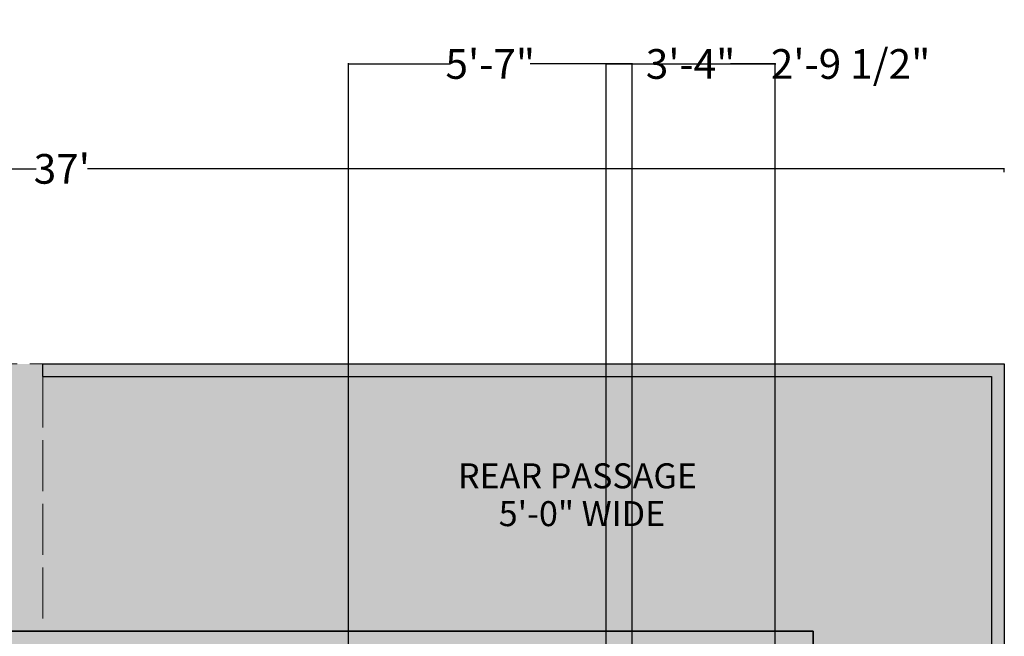
# Model space of a CAD drawing. Units: inches. Extents: x 1884 to 2398, y 474 to 1488.
# Tile 39 of 39: x 2165 to 2397, y 1343 to 1488. Entities that reach past the tile are written whole.
import ezdxf

# ---------------------------------------------------------------- set-up
doc = ezdxf.new("R2010")
doc.units = ezdxf.units.IN
doc.header["$MEASUREMENT"] = 0
doc.linetypes.add('ACAD_ISO02W100', pattern=[15, 12, -3])
for name, color, linetype, lineweight in [('A-ANNO-DIMS', 2, 'Continuous', 18), ('A-AREA-IDEN', 7, 'Continuous', 18), ('A-FLOR-OVHD', 8, 'ACAD_ISO02W100', 18), ('A-FLOR-PATT', 254, 'Continuous', 13), ('A-WALL-PATT', 250, 'Continuous', 13), ('C-PROP', 7, 'Continuous', 30), ('walls', 7, 'Continuous', 35)]:
    doc.layers.add(name, color=color, linetype=linetype, lineweight=lineweight)
doc.layers.add('L-PVMT-PATT', color=9, linetype='Continuous', lineweight=13, true_color=0xc7c8ca)
doc.styles.get("Standard").update_dxf_attribs({"font": 'arial.ttf'})
doc.dimstyles.get("Standard").update_dxf_attribs({"dimtxt": 7, "dimasz": 0.18, "dimexe": 0.18, "dimexo": 0.0625, "dimgap": 0.09, "dimtad": 0, "dimtih": 1, "dimtoh": 1, "dimzin": 0, "dimdsep": 46, "dimlunit": 3, "dimtxsty": 'Standard', "dimcen": 0.09, "dimadec": 0, "dimazin": 0, "dimtfac": 1, "dimtofl": 0, "dimtmove": 0, "dimatfit": 3, "dimfxl": 1, "dimtolj": 1, "dimtzin": 0, "dimarcsym": 0})

# ---------------------------------------------------------------- blocks, each defined once
blk = doc.blocks.new('*D1')
at = {"layer": 'A-ANNO-DIMS', "color": 0, "lineweight": -2, "transparency": 16777216}
for p, q in [((1952.53, 1452.05), (1952.53, 1453.03)), ((1952.71, 1452.85), (2168.5, 1452.85)), ((2396.35, 1452.85), (2180.56, 1452.85)), ((2396.53, 1452.05), (2396.53, 1453.03))]:
    blk.add_line(p, q, dxfattribs=at)
at = {"layer": 'A-ANNO-DIMS', "color": 0, "lineweight": 100, "transparency": 16777216}
for points in [[(1952.71, 1452.88), (1952.71, 1452.82), (1952.53, 1452.85)], [(2396.35, 1452.88), (2396.35, 1452.82), (2396.53, 1452.85)]]:
    blk.add_solid(points, dxfattribs=at)
at = {"layer": 'Defpoints', "color": 0, "lineweight": 100, "transparency": 16777216}
for p in [(1952.53, 1451.98), (2396.53, 1452.85), (2396.53, 1451.98)]:
    blk.add_point(p, dxfattribs=at)
at = {"layer": 'A-ANNO-DIMS', "color": 0, "transparency": 16777216, "insert": (2174.53, 1452.85), "char_height": 7, "attachment_point": 5}
blk.add_mtext("\\A1;37'", dxfattribs=at)
blk = doc.blocks.new('*D43')
at = {"layer": 'A-ANNO-DIMS', "color": 0, "lineweight": -2, "transparency": 16777216}
for p, q in [((2302.73, 1334.95), (2302.73, 1477.76)), ((2302.91, 1477.58), (2313.24, 1477.58)), ((2342.35, 1477.58), (2332.02, 1477.58)), ((2342.53, 1334.95), (2342.53, 1477.76))]:
    blk.add_line(p, q, dxfattribs=at)
at = {"layer": 'A-ANNO-DIMS', "color": 0, "lineweight": 100, "transparency": 16777216}
for points in [[(2302.91, 1477.61), (2302.91, 1477.55), (2302.73, 1477.58)], [(2342.35, 1477.61), (2342.35, 1477.55), (2342.53, 1477.58)]]:
    blk.add_solid(points, dxfattribs=at)
at = {"layer": 'Defpoints', "color": 0, "lineweight": 100, "transparency": 16777216}
for p in [(2342.53, 1477.58), (2302.73, 1334.88), (2342.53, 1334.88)]:
    blk.add_point(p, dxfattribs=at)
at = {"layer": 'A-ANNO-DIMS', "color": 0, "transparency": 16777216, "insert": (2322.63, 1477.58), "char_height": 7, "attachment_point": 5}
blk.add_mtext('\\A1;3\'-4"', dxfattribs=at)
blk = doc.blocks.new('*D52')
at = {"layer": 'A-ANNO-DIMS', "color": 0, "lineweight": -2, "transparency": 16777216}
for p, q in [((2308.85, 820.89), (2308.85, 1477.76)), ((2309.03, 1477.58), (2342.35, 1477.58)), ((2342.53, 820.89), (2342.53, 1477.76)), ((2342.53, 1477.58), (2342.71, 1477.58))]:
    blk.add_line(p, q, dxfattribs=at)
at = {"layer": 'A-ANNO-DIMS', "color": 0, "lineweight": 100, "transparency": 16777216}
for points in [[(2309.03, 1477.61), (2309.03, 1477.55), (2308.85, 1477.58)], [(2342.35, 1477.61), (2342.35, 1477.55), (2342.53, 1477.58)]]:
    blk.add_solid(points, dxfattribs=at)
at = {"layer": 'Defpoints', "color": 0, "lineweight": 100, "transparency": 16777216}
for p in [(2342.53, 1477.58), (2308.85, 820.83), (2342.53, 820.83)]:
    blk.add_point(p, dxfattribs=at)
at = {"layer": 'A-ANNO-DIMS', "color": 0, "transparency": 16777216, "insert": (2360.32, 1477.58), "char_height": 7, "attachment_point": 5}
blk.add_mtext('\\A1;2\'-9 1/2"', dxfattribs=at)
blk = doc.blocks.new('*D54')
at = {"layer": 'A-ANNO-DIMS', "color": 0, "lineweight": -2, "transparency": 16777216}
for p, q in [((2242.06, 893.03), (2242.06, 1477.76)), ((2242.24, 1477.58), (2266.06, 1477.58)), ((2308.67, 1477.58), (2284.85, 1477.58)), ((2308.85, 893.03), (2308.85, 1477.76))]:
    blk.add_line(p, q, dxfattribs=at)
at = {"layer": 'A-ANNO-DIMS', "color": 0, "lineweight": 100, "transparency": 16777216}
for points in [[(2242.24, 1477.61), (2242.24, 1477.55), (2242.06, 1477.58)], [(2308.67, 1477.61), (2308.67, 1477.55), (2308.85, 1477.58)]]:
    blk.add_solid(points, dxfattribs=at)
at = {"layer": 'Defpoints', "color": 0, "lineweight": 100, "transparency": 16777216}
for p in [(2308.85, 1477.58), (2242.06, 892.97), (2308.85, 892.97)]:
    blk.add_point(p, dxfattribs=at)
at = {"layer": 'A-ANNO-DIMS', "color": 0, "transparency": 16777216, "insert": (2275.45, 1477.58), "char_height": 7, "attachment_point": 5}
blk.add_mtext('\\A1;5\'-7"', dxfattribs=at)

msp = doc.modelspace()

# ---------------------------------------------------------------- hatches: boundary and pattern name
at = {"layer": 'A-FLOR-PATT'}
h = msp.add_hatch(color=256, dxfattribs=at)
h.dxf.hatch_style = 1
h.paths.add_polyline_path([(2170.029, 1403.885), (2170.029, 1406.885), (2092.029, 1406.885), (2092.029, 1328.623), (2148.233, 1328.623), (2158.029, 1328.623), (2158.029, 1334.885), (2158.029, 1343.885), (2164.726, 1343.885), (2170.029, 1343.885)])
at = {"layer": 'A-WALL-PATT'}
h = msp.add_hatch(color=256, dxfattribs=at)
h.dxf.hatch_style = 1
h.paths.add_polyline_path([(2092.029, 1406.885), (1952.529, 1406.885), (1952.529, 939.249), (1955.529, 939.249), (1955.529, 1069.385), (1969.695, 1069.385), (1969.695, 1078.385), (1961.529, 1078.385), (1961.529, 1397.885), (2087.529, 1397.885), (2087.529, 1322.885), (2092.029, 1322.885), (2092.029, 1328.623)])
h.paths.add_polyline_path([(2087.529, 1345.919), (2014.612, 1345.919), (2014.612, 1327.385), (2007.132, 1327.385), (2007.132, 1322.885), (2019.112, 1322.885), (2019.112, 1327.385), (2019.112, 1341.419), (2087.529, 1341.419)], flags=17)
h.paths.add_polyline_path([(1965.066, 1327.561), (1961.529, 1327.561), (1961.529, 1322.885), (1965.066, 1322.885)], flags=17)
h.paths.add_polyline_path([(2351.529, 1343.885), (2265.892, 1343.885), (2164.726, 1343.885), (2158.029, 1343.885), (2158.029, 1334.885), (2158.029, 1328.623), (2148.233, 1328.623), (2148.233, 1322.885), (2158.029, 1322.885), (2158.029, 1276.197), (2158.029, 1166.885), (2152.638, 1166.885), (2152.638, 1157.885), (2158.029, 1157.885), (2158.029, 1104.929), (2168.6, 1104.929), (2168.6, 1247.885), (2209.755, 1247.885), (2209.755, 1252.385), (2167.029, 1252.385), (2167.029, 1334.885), (2265.892, 1334.885), (2342.529, 1334.885), (2342.529, 1310.041), (2351.529, 1310.041)])
h.paths.add_polyline_path([(2234.529, 1334.885), (2230.029, 1334.885), (2230.029, 1275.554), (2234.529, 1275.554)], flags=17)
h.paths.add_polyline_path([(2342.529, 1252.385), (2265.892, 1252.385), (2234.529, 1252.385), (2234.529, 1256.117), (2230.029, 1256.117), (2230.029, 1247.885), (2265.892, 1247.885), (2342.529, 1247.885)], flags=17)
h.paths.add_polyline_path([(2351.529, 1276.197), (2351.529, 1293.635), (2342.529, 1293.635), (2342.529, 1252.385), (2342.529, 1225.302), (2346.311, 1225.302), (2351.529, 1225.302)], flags=17)
h.paths.add_polyline_path([(2351.529, 1126.264), (2342.529, 1126.264), (2342.529, 1093.809), (2342.529, 1062.466), (2168.6, 1062.466), (2168.6, 1079.411), (2158.029, 1079.411), (2158.029, 1056.803), (2158.029, 1053.466), (2213.529, 1053.466), (2213.529, 934.675), (2222.529, 934.675), (2222.529, 1057.966), (2342.529, 1057.966), (2342.529, 1027.206), (2345.987, 1027.206), (2351.529, 1027.206)])
h.paths.add_polyline_path([(2116.005, 1166.885), (1961.529, 1166.885), (1961.529, 1162.385), (2081.529, 1162.385), (2081.529, 1152.292), (2090.529, 1152.292), (2090.529, 1157.885), (2116.005, 1157.885)])
h.paths.add_polyline_path([(2090.529, 1122.635), (2081.529, 1122.635), (2081.529, 1078.385), (2000.529, 1078.385), (2000.529, 1069.385), (2000.529, 1034.463), (2003.893, 1034.463), (2009.529, 1034.463), (2009.529, 1069.385), (2090.529, 1069.385)], flags=17)
h.paths.add_polyline_path([(2351.529, 974.676), (2342.529, 974.676), (2342.529, 951.86), (2351.529, 951.86)], flags=17)
h = msp.add_hatch(color=256, dxfattribs=at)
h.dxf.hatch_style = 1
h.paths.add_polyline_path([(2393.529, 1406.885), (2170.029, 1406.885), (2170.029, 1403.885), (2393.529, 1403.885)])
h = msp.add_hatch(color=256, dxfattribs=at)
h.dxf.hatch_style = 1
h.paths.add_polyline_path([(2396.529, 1406.885), (2393.529, 1406.885), (2393.529, 1061.532), (2396.529, 1061.532)])
h = msp.add_hatch(color=256, dxfattribs=at)
h.dxf.hatch_style = 1
h.paths.add_polyline_path([(2396.529, 1406.885), (2393.529, 1406.885), (2393.529, 779.322), (2396.529, 779.322)])
at = {"layer": 'L-PVMT-PATT'}
h = msp.add_hatch(color=256, dxfattribs=at)
h.dxf.hatch_style = 1
h.paths.add_polyline_path([(2393.529, 1403.885), (2170.029, 1403.885), (2170.029, 1343.885), (2265.892, 1343.885), (2351.529, 1343.885), (2351.529, 1276.197), (2351.529, 1062.466), (2369.436, 1062.466), (2369.436, 893.06), (2351.529, 893.06), (2351.529, 880.385), (2351.529, 779.322), (2387.529, 779.322), (2393.529, 779.322)])

# ---------------------------------------------------------------- linework, layer by layer
at = {"layer": 'A-FLOR-OVHD'}
for p, q in [((2092.029, 1406.885), (2170.029, 1406.885)), ((2170.029, 1403.885), (2170.029, 1343.885))]:
    msp.add_line(p, q, dxfattribs=at)
at = {"layer": 'C-PROP'}
for p, q in [((2170.029, 1406.885), (2396.529, 1406.885)), ((2170.029, 1403.885), (2170.029, 1406.885)), ((2396.529, 1406.885), (2396.529, 530.885)), ((2170.029, 1403.885), (2393.529, 1403.885)), ((2393.529, 1403.885), (2393.529, 779.322))]:
    msp.add_line(p, q, dxfattribs=at)
at = {"layer": 'walls'}
for p, q in [((2158.029, 1343.885), (2164.726, 1343.885)), ((2265.892, 1343.885), (2164.726, 1343.885)), ((2351.529, 1343.885), (2265.892, 1343.885)), ((2351.529, 1276.197), (2351.529, 1343.885))]:
    msp.add_line(p, q, dxfattribs=at)

# ---------------------------------------------------------------- texts
at = {"layer": 'A-AREA-IDEN'}
for s, height, p in [('REAR PASSAGE', 5.88789, (2267.835, 1377.544)), ('5\'-0" WIDE', 5.8879, (2277.438, 1368.627))]:
    msp.add_text(s, height=height, dxfattribs=at).set_placement(p)

# ---------------------------------------------------------------- dimensions: what is measured, and where the dimension line sits
at = {"layer": 'A-ANNO-DIMS'}
for base, p1, p2, override, picture, middle in [((2342.529, 1477.585), (2308.846, 820.826), (2342.529, 820.826), {"dimdec": 1, "dimlfac": 1, "dimrnd": 0, "dimzin": 1, "dimdsep": 46, "dimlunit": 4, "dimfrac": 2}, '*D52', (2360.318, 1477.585)), ((2308.846, 1477.585), (2242.059, 892.966), (2308.846, 892.966), {"dimdec": 1, "dimlfac": 1, "dimrnd": 0, "dimzin": 1, "dimdsep": 46, "dimlunit": 4, "dimfrac": 2}, '*D54', (2275.452, 1477.585)), ((2342.529, 1477.585), (2302.733, 1334.885), (2342.529, 1334.885), {"dimdec": 1, "dimlfac": 1, "dimrnd": 0, "dimzin": 1, "dimdsep": 46, "dimlunit": 4, "dimfrac": 2}, '*D43', (2322.631, 1477.585)), ((2396.529, 1452.853), (1952.529, 1451.984), (2396.529, 1451.984), {"dimclrd": 0, "dimclre": 0, "dimclrt": 0}, '*D1', (2174.529, 1452.853))]:
    dim = msp.add_linear_dim(base=base, p1=p1, p2=p2, dimstyle='Standard', override=override, dxfattribs=at)
    dim.commit()
    dim.dimension.update_dxf_attribs({"geometry": picture, "text_midpoint": middle})

doc.saveas('drawing.dxf')
